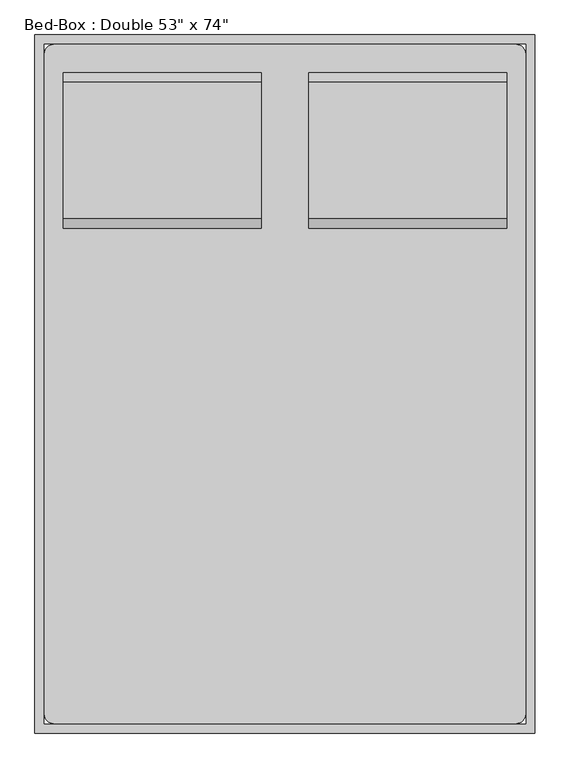
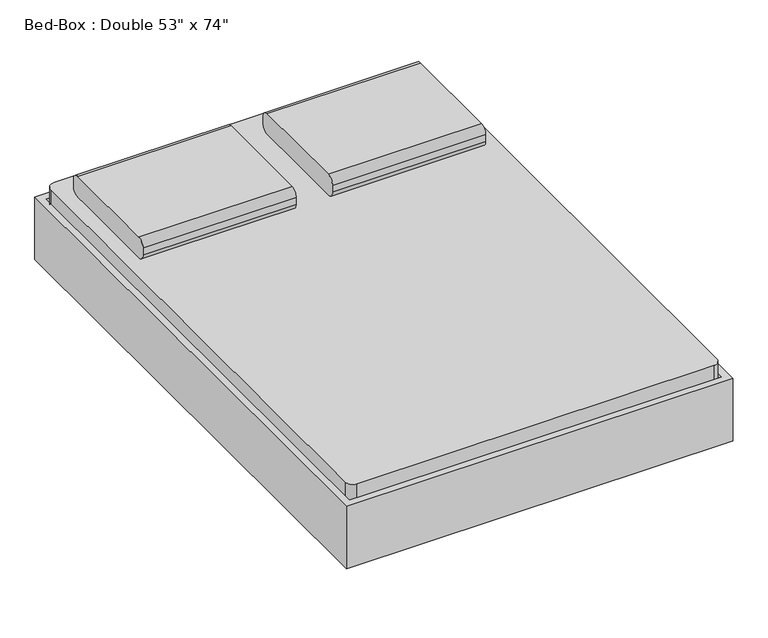
"""IFC4 building model written with IfcOpenShell, lengths in millimetres: furniture geometry."""

from ifc_helpers import new_model, si_unit, point, frame, frame_2d, origin, place, context, project, spatial, polyline, circle_curve, trimmed, segment, composite_curve, outline, extrude, source, transform, mapped, element, save
from ifc_brep_helpers import plane_surface, cylinder_surface, revolved_surface, advanced_brep


def furniture_c8abb964(model_context):
    return source(origin(), model_context, "Body", "SolidModel", [
        extrude(outline(composite_curve([segment(polyline([(578.3704918, 406.4), (210.0704918, 406.4)]), True, "CONTINUOUS"), segment(trimmed(circle_curve(frame_2d((210.0704918, 431.8)), 25.4), [point((210.0704918, 406.4))], [point((184.6704918, 431.8))], False, "CARTESIAN"), True, "CONTINUOUS"), segment(polyline([(184.6704918, 431.8), (184.6704918, 457.2)]), True, "CONTINUOUS"), segment(trimmed(circle_curve(frame_2d((210.0704918, 457.2)), 25.4), [point((184.6704918, 457.2))], [point((210.0704918, 482.6))], False, "CARTESIAN"), True, "CONTINUOUS"), segment(polyline([(210.0704918, 482.6), (578.3704918, 482.6)]), True, "CONTINUOUS"), segment(trimmed(circle_curve(frame_2d((578.3704918, 457.2)), 25.4), [point((578.3704918, 482.6))], [point((603.7704918, 457.2))], False, "CARTESIAN"), True, "CONTINUOUS"), segment(polyline([(603.7704918, 457.2), (603.7704918, 431.8)]), True, "CONTINUOUS"), segment(trimmed(circle_curve(frame_2d((578.3704918, 431.8)), 25.4), [point((603.7704918, 431.8))], [point((578.3704918, 406.4))], False, "CARTESIAN"), True, "CONTINUOUS")], self_intersect=False)), frame((402.652459, 0.0, 0.0), z_axis=(1.0, 0.0, 0.0), x_axis=(0.0, 1.0, 0.0)), (0.0, 0.0, 1.0), 533.4),
        extrude(outline(composite_curve([segment(polyline([(578.3704918, 406.4), (210.0704918, 406.4)]), True, "CONTINUOUS"), segment(trimmed(circle_curve(frame_2d((210.0704918, 431.8)), 25.4), [point((210.0704918, 406.4))], [point((184.6704918, 431.8))], False, "CARTESIAN"), True, "CONTINUOUS"), segment(polyline([(184.6704918, 431.8), (184.6704918, 457.2)]), True, "CONTINUOUS"), segment(trimmed(circle_curve(frame_2d((210.0704918, 457.2)), 25.4), [point((184.6704918, 457.2))], [point((210.0704918, 482.6))], False, "CARTESIAN"), True, "CONTINUOUS"), segment(polyline([(210.0704918, 482.6), (578.3704918, 482.6)]), True, "CONTINUOUS"), segment(trimmed(circle_curve(frame_2d((578.3704918, 457.2)), 25.4), [point((578.3704918, 482.6))], [point((603.7704918, 457.2))], False, "CARTESIAN"), True, "CONTINUOUS"), segment(polyline([(603.7704918, 457.2), (603.7704918, 431.8)]), True, "CONTINUOUS"), segment(trimmed(circle_curve(frame_2d((578.3704918, 431.8)), 25.4), [point((603.7704918, 431.8))], [point((578.3704918, 406.4))], False, "CARTESIAN"), True, "CONTINUOUS")], self_intersect=False)), frame((-257.747541, 0.0, 0.0), z_axis=(1.0, 0.0, 0.0), x_axis=(0.0, 1.0, 0.0)), (0.0, 0.0, 1.0), 533.4),
        advanced_brep(
        [(-308.2231784, 451.3704918, 177.8), (-308.2231784, 375.1704918, 177.8), (-308.2231784, 375.1704918, 196.85), (-308.2231784, 451.3704918, 196.85), (-257.4231784, 451.3704918, 177.8), (-257.4231784, 375.1704918, 177.8), (-245.2869899, 375.1704918, 196.85), (-245.2869899, 451.3704918, 196.85), (-181.3523099, 451.3704918, 14.6654962), (-181.3523099, 375.1704918, 14.6654962), (-164.0871466, 375.1704918, 22.716374), (-164.0871466, 451.3704918, 22.716374), (-158.3320921, 375.1704918, 0.0), (-158.3320921, 451.3704918, 0.0), (-158.3320921, 375.1704918, 19.05), (-158.3320921, 451.3704918, 19.05), (-79.7195862, 451.3704918, 0.0), (-79.7195862, 375.1704918, 0.0), (-79.7195862, 375.1704918, 19.05), (-79.7195862, 451.3704918, 19.05), (-67.0195862, 375.1704918, 3.4029547), (-67.0195862, 451.3704918, 3.4029547), (-76.5445862, 375.1704918, 19.9007387), (-76.5445862, 451.3704918, 19.9007387), (-6.922541, 451.3704918, 38.1), (-6.922541, 375.1704918, 38.1), (-12.0269731, 375.1704918, 57.15), (-12.0269731, 451.3704918, 57.15), (685.5518216, 451.3704918, 38.1), (685.5518216, 375.1704918, 38.1), (690.6562537, 375.1704918, 57.15), (690.6562537, 451.3704918, 57.15), (745.6488669, 451.3704918, 3.4029547), (745.6488669, 375.1704918, 3.4029547), (755.1738669, 375.1704918, 19.9007387), (755.1738669, 451.3704918, 19.9007387), (758.3488669, 375.1704918, 0.0), (758.3488669, 451.3704918, 0.0), (758.3488669, 375.1704918, 19.05), (758.3488669, 451.3704918, 19.05), (836.9613728, 451.3704918, 0.0), (836.9613728, 375.1704918, 0.0), (836.9613728, 375.1704918, 19.05), (836.9613728, 451.3704918, 19.05), (859.9815906, 375.1704918, 14.6654962), (859.9815906, 451.3704918, 14.6654962), (842.7164272, 375.1704918, 22.716374), (842.7164272, 451.3704918, 22.716374), (936.052459, 451.3704918, 177.8), (936.052459, 375.1704918, 177.8), (923.9162705, 375.1704918, 196.85), (923.9162705, 451.3704918, 196.85), (986.852459, 451.3704918, 177.8), (986.852459, 451.3704918, 196.85), (986.852459, 375.1704918, 196.85), (986.852459, 375.1704918, 177.8)],
        [
            (0, 1),
            (1, 2),
            (2, 3),
            (3, 0),
            (0, 4),
            (4, 5),
            (5, 1),
            (5, 6),
            (6, 2),
            (6, 7),
            (7, 3),
            (7, 4),
            (4, 8),
            (8, 9),
            (9, 5),
            (9, 10),
            (10, 6),
            (10, 11),
            (11, 7),
            (11, 8),
            (12, 9, circle_curve(frame((-158.3320921, 375.1704918, 25.4), z_axis=(0.0, 1.0, 0.0), x_axis=(-0.9063077870366486, 0.0, -0.42261826174070233)), 25.4)),
            (8, 13, circle_curve(frame((-158.3320921, 451.3704918, 25.4), z_axis=(0.0, -1.0, 0.0), x_axis=(-0.9063077870366486, 0.0, -0.42261826174070233)), 25.4)),
            (13, 12),
            (14, 10, circle_curve(frame((-158.3320921, 375.1704918, 25.4), z_axis=(0.0, 1.0, 0.0), x_axis=(-0.9063077870366486, 0.0, -0.42261826174070233)), 6.35)),
            (12, 14),
            (15, 11, circle_curve(frame((-158.3320921, 451.3704918, 25.4), z_axis=(0.0, 1.0, 0.0), x_axis=(-0.9063077870366486, 0.0, -0.42261826174070233)), 6.35)),
            (14, 15),
            (15, 13),
            (13, 16),
            (16, 17),
            (17, 12),
            (17, 18),
            (18, 14),
            (18, 19),
            (19, 15),
            (19, 16),
            (20, 17, circle_curve(frame((-79.7195862, 375.1704918, 25.4), z_axis=(0.0, 1.0, 0.0), x_axis=(0.0, 0.0, -1.0)), 25.4)),
            (16, 21, circle_curve(frame((-79.7195862, 451.3704918, 25.4), z_axis=(0.0, -1.0, 0.0), x_axis=(0.0, 0.0, -1.0)), 25.4)),
            (21, 20),
            (22, 18, circle_curve(frame((-79.7195862, 375.1704918, 25.4), z_axis=(0.0, 1.0, 0.0), x_axis=(0.0, 0.0, -1.0)), 6.35)),
            (20, 22),
            (23, 19, circle_curve(frame((-79.7195862, 451.3704918, 25.4), z_axis=(0.0, 1.0, 0.0), x_axis=(0.0, 0.0, -1.0)), 6.35)),
            (22, 23),
            (23, 21),
            (21, 24),
            (24, 25),
            (25, 20),
            (25, 26),
            (26, 22),
            (26, 27),
            (27, 23),
            (27, 24),
            (24, 28),
            (28, 29),
            (29, 25),
            (29, 30),
            (30, 26),
            (30, 31),
            (31, 27),
            (31, 28),
            (28, 32),
            (32, 33),
            (33, 29),
            (33, 34),
            (34, 30),
            (34, 35),
            (35, 31),
            (35, 32),
            (36, 33, circle_curve(frame((758.3488669, 375.1704918, 25.4), z_axis=(0.0, 1.0, 0.0), x_axis=(-0.5000000000000463, 0.0, -0.8660254037844118)), 25.4)),
            (32, 37, circle_curve(frame((758.3488669, 451.3704918, 25.4), z_axis=(0.0, -1.0, 0.0), x_axis=(-0.5000000000000463, 0.0, -0.8660254037844118)), 25.4)),
            (37, 36),
            (38, 34, circle_curve(frame((758.3488669, 375.1704918, 25.4), z_axis=(0.0, 1.0, 0.0), x_axis=(-0.5000000000000463, 0.0, -0.8660254037844118)), 6.35)),
            (36, 38),
            (39, 35, circle_curve(frame((758.3488669, 451.3704918, 25.4), z_axis=(0.0, 1.0, 0.0), x_axis=(-0.5000000000000463, 0.0, -0.8660254037844118)), 6.35)),
            (38, 39),
            (39, 37),
            (37, 40),
            (40, 41),
            (41, 36),
            (41, 42),
            (42, 38),
            (42, 43),
            (43, 39),
            (43, 40),
            (44, 41, circle_curve(frame((836.9613728, 375.1704918, 25.4), z_axis=(0.0, 1.0, 0.0), x_axis=(0.0, 0.0, -1.0)), 25.4)),
            (40, 45, circle_curve(frame((836.9613728, 451.3704918, 25.4), z_axis=(0.0, -1.0, 0.0), x_axis=(0.0, 0.0, -1.0)), 25.4)),
            (45, 44),
            (46, 42, circle_curve(frame((836.9613728, 375.1704918, 25.4), z_axis=(0.0, 1.0, 0.0), x_axis=(0.0, 0.0, -1.0)), 6.35)),
            (44, 46),
            (47, 43, circle_curve(frame((836.9613728, 451.3704918, 25.4), z_axis=(0.0, 1.0, 0.0), x_axis=(0.0, 0.0, -1.0)), 6.35)),
            (46, 47),
            (47, 45),
            (45, 48),
            (48, 49),
            (49, 44),
            (49, 50),
            (50, 46),
            (50, 51),
            (51, 47),
            (51, 48),
            (52, 53),
            (53, 54),
            (54, 55),
            (55, 52),
            (48, 52),
            (55, 49),
            (54, 50),
            (53, 51),
        ],
        [
            plane_surface(frame((-308.2231784, 705.3704918, -152.9490627), z_axis=(-1.0, 0.0, 0.0), x_axis=(0.0, 1.0, 0.0))),
            plane_surface(frame((-308.2231784, 451.3704918, 177.8), z_axis=(0.0, 0.0, -1.0), x_axis=(1.0, 0.0, 0.0))),
            plane_surface(frame((-308.2231784, 375.1704918, 177.8), z_axis=(0.0, -1.0, 0.0), x_axis=(1.0, 0.0, 0.0))),
            plane_surface(frame((-308.2231784, 375.1704918, 196.85), z_axis=(0.0, 0.0, 1.0), x_axis=(1.0, 0.0, 0.0))),
            plane_surface(frame((-308.2231784, 451.3704918, 196.85), z_axis=(0.0, 1.0, 0.0), x_axis=(1.0, 0.0, 0.0))),
            plane_surface(frame((-257.4231784, 451.3704918, 177.8), z_axis=(-0.9063077870366488, 0.0, -0.42261826174070194), x_axis=(0.42261826174070194, 0.0, -0.9063077870366488))),
            plane_surface(frame((-257.4231784, 375.1704918, 177.8), z_axis=(0.0, -1.0, 0.0), x_axis=(0.42261826174070194, 0.0, -0.9063077870366488))),
            plane_surface(frame((-245.2869899, 375.1704918, 196.85), z_axis=(0.9063077870366487, 0.0, 0.4226182617407021), x_axis=(0.4226182617407021, 0.0, -0.9063077870366487))),
            plane_surface(frame((-245.2869899, 451.3704918, 196.85), z_axis=(0.0, 1.0, 0.0), x_axis=(0.4226182617407021, 0.0, -0.9063077870366487))),
            cylinder_surface(frame((-158.3320921, 705.3704918, 25.4), z_axis=(0.0, -1.0, 0.0), x_axis=(-0.9063077870366486, 0.0, -0.42261826174070233)), 25.4),
            plane_surface(frame((-158.3320921, 375.1704918, 25.4), z_axis=(0.0, -1.0, 0.0), x_axis=(-0.9063077870366486, 0.0, -0.42261826174070233))),
            revolved_surface(polyline([(-164.08714654768272, 375.1704918, 22.71637403794654), (-164.08714654768272, 451.3704918, 22.71637403794654)]), (-158.3320921, 705.3704918, 25.4), (0.0, -1.0, 0.0)),
            plane_surface(frame((-158.3320921, 451.3704918, 25.4), z_axis=(0.0, 1.0, 0.0), x_axis=(-0.9063077870366486, 0.0, -0.42261826174070233))),
            plane_surface(frame((-158.3320921, 451.3704918, 0.0), z_axis=(0.0, 0.0, -1.0), x_axis=(1.0, 0.0, 0.0))),
            plane_surface(frame((-158.3320921, 375.1704918, 0.0), z_axis=(0.0, -1.0, 0.0), x_axis=(1.0, 0.0, 0.0))),
            plane_surface(frame((-158.3320921, 375.1704918, 19.05), z_axis=(0.0, 0.0, 1.0), x_axis=(1.0, 0.0, 0.0))),
            plane_surface(frame((-158.3320921, 451.3704918, 19.05), z_axis=(0.0, 1.0, 0.0), x_axis=(1.0, 0.0, 0.0))),
            cylinder_surface(frame((-79.7195862, 705.3704918, 25.4), z_axis=(0.0, -1.0, 0.0), x_axis=(0.0, 0.0, -1.0)), 25.4),
            plane_surface(frame((-79.7195862, 375.1704918, 25.4), z_axis=(0.0, -1.0, 0.0), x_axis=(0.0, 0.0, -1.0))),
            revolved_surface(polyline([(-79.7195862, 375.1704918, 19.049999999999997), (-79.7195862, 451.3704918, 19.049999999999997)]), (-79.7195862, 705.3704918, 25.4), (0.0, -1.0, 0.0)),
            plane_surface(frame((-79.7195862, 451.3704918, 25.4), z_axis=(0.0, 1.0, 0.0), x_axis=(0.0, 0.0, -1.0))),
            plane_surface(frame((-67.0195862, 451.3704918, 3.4029547), z_axis=(0.4999999999998775, 0.0, -0.8660254037845094), x_axis=(0.8660254037845094, 0.0, 0.4999999999998775))),
            plane_surface(frame((-67.0195862, 375.1704918, 3.4029547), z_axis=(0.0, -1.0, 0.0), x_axis=(0.866025403784509, 0.0, 0.49999999999987826))),
            plane_surface(frame((-76.5445862, 375.1704918, 19.9007387), z_axis=(-0.49999999999987754, 0.0, 0.8660254037845093), x_axis=(0.8660254037845093, 0.0, 0.49999999999987754))),
            plane_surface(frame((-76.5445862, 451.3704918, 19.9007387), z_axis=(0.0, 1.0000000000000002, 0.0), x_axis=(0.8660254037845091, 0.0, 0.49999999999987815))),
            plane_surface(frame((-6.922541, 451.3704918, 38.1), z_axis=(0.0, 0.0, -1.0), x_axis=(1.0, 0.0, 0.0))),
            plane_surface(frame((-6.922541, 375.1704918, 38.1), z_axis=(0.0, -1.0, 0.0), x_axis=(1.0, 0.0, 0.0))),
            plane_surface(frame((-12.0269731, 375.1704918, 57.15), z_axis=(0.0, 0.0, 1.0), x_axis=(1.0, 0.0, 0.0))),
            plane_surface(frame((-12.0269731, 451.3704918, 57.15), z_axis=(0.0, 1.0, 0.0), x_axis=(1.0, 0.0, 0.0))),
            plane_surface(frame((685.5518216, 451.3704918, 38.1), z_axis=(-0.500000000000047, 0.0, -0.8660254037844116), x_axis=(0.8660254037844116, 0.0, -0.500000000000047))),
            plane_surface(frame((685.5518216, 375.1704918, 38.1), z_axis=(0.0, -1.0, 0.0), x_axis=(0.8660254037844122, 0.0, -0.5000000000000459))),
            plane_surface(frame((690.6562537, 375.1704918, 57.15), z_axis=(0.5000000000000461, 0.0, 0.8660254037844121), x_axis=(0.8660254037844121, 0.0, -0.5000000000000461))),
            plane_surface(frame((690.6562537, 451.3704918, 57.15), z_axis=(0.0, 1.0, 0.0), x_axis=(0.8660254037844127, 0.0, -0.500000000000045))),
            cylinder_surface(frame((758.3488669, 705.3704918, 25.4), z_axis=(0.0, -1.0, 0.0), x_axis=(-0.5000000000000463, 0.0, -0.8660254037844118)), 25.4),
            plane_surface(frame((758.3488669, 375.1704918, 25.4), z_axis=(0.0, -1.0000000000000002, 0.0), x_axis=(-0.5000000000000464, 0.0, -0.866025403784412))),
            revolved_surface(polyline([(755.1738668999997, 375.1704918, 19.90073868596898), (755.1738668999997, 451.3704918, 19.90073868596898)]), (758.3488669, 705.3704918, 25.4), (0.0, -1.0, 0.0)),
            plane_surface(frame((758.3488669, 451.3704918, 25.4), z_axis=(0.0, 1.0000000000000002, 0.0), x_axis=(-0.5000000000000464, 0.0, -0.866025403784412))),
            plane_surface(frame((758.3488669, 451.3704918, 0.0), z_axis=(0.0, 0.0, -1.0), x_axis=(1.0, 0.0, 0.0))),
            plane_surface(frame((758.3488669, 375.1704918, 0.0), z_axis=(0.0, -1.0, 0.0), x_axis=(1.0, 0.0, 0.0))),
            plane_surface(frame((758.3488669, 375.1704918, 19.05), z_axis=(0.0, 0.0, 1.0), x_axis=(1.0, 0.0, 0.0))),
            plane_surface(frame((758.3488669, 451.3704918, 19.05), z_axis=(0.0, 1.0, 0.0), x_axis=(1.0, 0.0, 0.0))),
            cylinder_surface(frame((836.9613728, 705.3704918, 25.4), z_axis=(0.0, -1.0, 0.0), x_axis=(0.0, 0.0, -1.0)), 25.4),
            plane_surface(frame((836.9613728, 375.1704918, 25.4), z_axis=(0.0, -1.0, 0.0), x_axis=(0.0, 0.0, -1.0))),
            revolved_surface(polyline([(836.9613728, 375.1704918, 19.049999999999997), (836.9613728, 451.3704918, 19.049999999999997)]), (836.9613728, 705.3704918, 25.4), (0.0, -1.0, 0.0)),
            plane_surface(frame((836.9613728, 451.3704918, 25.4), z_axis=(0.0, 1.0, 0.0), x_axis=(0.0, 0.0, -1.0))),
            plane_surface(frame((859.9815906, 451.3704918, 14.6654962), z_axis=(0.9063077870366797, 0.0, -0.42261826174063566), x_axis=(0.42261826174063566, 0.0, 0.9063077870366797))),
            plane_surface(frame((859.9815906, 375.1704918, 14.6654962), z_axis=(0.0, -1.0000000000000002, 0.0), x_axis=(0.4226182617406349, 0.0, 0.9063077870366801))),
            plane_surface(frame((842.7164272, 375.1704918, 22.716374), z_axis=(-0.9063077870366799, 0.0, 0.4226182617406354), x_axis=(0.4226182617406354, 0.0, 0.9063077870366799))),
            plane_surface(frame((842.7164272, 451.3704918, 22.716374), z_axis=(0.0, 1.0, 0.0), x_axis=(0.42261826174063555, 0.0, 0.9063077870366798))),
            plane_surface(frame((986.852459, 705.3704918, -152.9490627), z_axis=(1.0, 0.0, 0.0), x_axis=(0.0, 1.0, 0.0))),
            plane_surface(frame((936.052459, 451.3704918, 177.8), z_axis=(0.0, 0.0, -1.0), x_axis=(1.0, 0.0, 0.0))),
            plane_surface(frame((936.052459, 375.1704918, 177.8), z_axis=(0.0, -1.0, 0.0), x_axis=(1.0, 0.0, 0.0))),
            plane_surface(frame((923.9162705, 375.1704918, 196.85), z_axis=(0.0, 0.0, 1.0), x_axis=(1.0, 0.0, 0.0))),
            plane_surface(frame((923.9162705, 451.3704918, 196.85), z_axis=(0.0, 1.0, 0.0), x_axis=(1.0, 0.0, 0.0))),
        ],
        [
            (0, [[1, 2, 3, 4]]),
            (1, [[-1, 5, 6, 7]]),
            (2, [[-2, -7, 8, 9]]),
            (3, [[-3, -9, 10, 11]]),
            (4, [[-4, -11, 12, -5]]),
            (5, [[-6, 13, 14, 15]]),
            (6, [[-8, -15, 16, 17]]),
            (7, [[-10, -17, 18, 19]]),
            (8, [[-12, -19, 20, -13]]),
            (9, [[21, -14, 22, 23]]),
            (10, [[24, -16, -21, 25]]),
            (11, [[26, -18, -24, 27]]),
            (12, [[-22, -20, -26, 28]]),
            (13, [[-23, 29, 30, 31]]),
            (14, [[-25, -31, 32, 33]]),
            (15, [[-27, -33, 34, 35]]),
            (16, [[-28, -35, 36, -29]]),
            (17, [[37, -30, 38, 39]]),
            (18, [[40, -32, -37, 41]]),
            (19, [[42, -34, -40, 43]]),
            (20, [[-38, -36, -42, 44]]),
            (21, [[-39, 45, 46, 47]]),
            (22, [[-41, -47, 48, 49]]),
            (23, [[-43, -49, 50, 51]]),
            (24, [[-44, -51, 52, -45]]),
            (25, [[-46, 53, 54, 55]]),
            (26, [[-48, -55, 56, 57]]),
            (27, [[-50, -57, 58, 59]]),
            (28, [[-52, -59, 60, -53]]),
            (29, [[-54, 61, 62, 63]]),
            (30, [[-56, -63, 64, 65]]),
            (31, [[-58, -65, 66, 67]]),
            (32, [[-60, -67, 68, -61]]),
            (33, [[69, -62, 70, 71]]),
            (34, [[72, -64, -69, 73]]),
            (35, [[74, -66, -72, 75]]),
            (36, [[-70, -68, -74, 76]]),
            (37, [[-71, 77, 78, 79]]),
            (38, [[-73, -79, 80, 81]]),
            (39, [[-75, -81, 82, 83]]),
            (40, [[-76, -83, 84, -77]]),
            (41, [[85, -78, 86, 87]]),
            (42, [[88, -80, -85, 89]]),
            (43, [[90, -82, -88, 91]]),
            (44, [[-86, -84, -90, 92]]),
            (45, [[-87, 93, 94, 95]]),
            (46, [[-89, -95, 96, 97]]),
            (47, [[-91, -97, 98, 99]]),
            (48, [[-92, -99, 100, -93]]),
            (49, [[101, 102, 103, 104]]),
            (50, [[-94, 105, -104, 106]]),
            (51, [[-96, -106, -103, 107]]),
            (52, [[-98, -107, -102, 108]]),
            (53, [[-100, -108, -101, -105]]),
        ],
    ),
        extrude(outline(composite_curve([segment(polyline([(-283.147541, 679.9704918), (961.452459, 679.9704918)]), True, "CONTINUOUS"), segment(trimmed(circle_curve(frame_2d((961.452459, 654.5704918)), 25.4), [point((961.452459, 679.9704918))], [point((986.852459, 654.5704918))], False, "CARTESIAN"), True, "CONTINUOUS"), segment(polyline([(986.852459, 654.5704918), (986.852459, -1123.4295082)]), True, "CONTINUOUS"), segment(trimmed(circle_curve(frame_2d((961.452459, -1123.4295082)), 25.4), [point((986.852459, -1123.4295082))], [point((961.452459, -1148.8295082))], False, "CARTESIAN"), True, "CONTINUOUS"), segment(polyline([(961.452459, -1148.8295082), (-283.147541, -1148.8295082)]), True, "CONTINUOUS"), segment(trimmed(circle_curve(frame_2d((-283.147541, -1123.4295082)), 25.4), [point((-283.147541, -1148.8295082))], [point((-308.547541, -1123.4295082))], False, "CARTESIAN"), True, "CONTINUOUS"), segment(polyline([(-308.547541, -1123.4295082), (-308.547541, 654.5704918)]), True, "CONTINUOUS"), segment(trimmed(circle_curve(frame_2d((-283.147541, 654.5704918)), 25.4), [point((-308.547541, 654.5704918))], [point((-283.147541, 679.9704918))], False, "CARTESIAN"), True, "CONTINUOUS")], self_intersect=False)), frame((0.0, 0.0, 203.2), z_axis=(0.0, 0.0, 1.0), x_axis=(1.0, 0.0, 0.0)), (0.0, 0.0, 1.0), 203.2),
        advanced_brep(
        [(-308.547541, -869.4295082, 196.85), (-308.547541, -869.4295082, 177.8), (-308.547541, -945.6295082, 177.8), (-308.547541, -945.6295082, 196.85), (-245.6113525, -869.4295082, 196.85), (-257.747541, -869.4295082, 177.8), (-257.747541, -945.6295082, 177.8), (-245.6113525, -945.6295082, 196.85), (-164.4115092, -869.4295082, 22.716374), (-181.6766725, -869.4295082, 14.6654962), (-181.6766725, -945.6295082, 14.6654962), (-164.4115092, -945.6295082, 22.716374), (-158.6564547, -869.4295082, 0.0), (-158.6564547, -869.4295082, 19.05), (-158.6564547, -945.6295082, 0.0), (-158.6564547, -945.6295082, 19.05), (-80.0439489, -869.4295082, 19.05), (-80.0439489, -869.4295082, 0.0), (-80.0439489, -945.6295082, 0.0), (-80.0439489, -945.6295082, 19.05), (-67.3439489, -869.4295082, 3.4029547), (-76.8689489, -869.4295082, 19.9007387), (-67.3439489, -945.6295082, 3.4029547), (-76.8689489, -945.6295082, 19.9007387), (-12.3513357, -869.4295082, 57.15), (-7.2469036, -869.4295082, 38.1), (-7.2469036, -945.6295082, 38.1), (-12.3513357, -945.6295082, 57.15), (690.6562537, -869.4295082, 57.15), (685.5518216, -869.4295082, 38.1), (685.5518216, -945.6295082, 38.1), (690.6562537, -945.6295082, 57.15), (755.1738669, -869.4295082, 19.9007387), (745.6488669, -869.4295082, 3.4029547), (745.6488669, -945.6295082, 3.4029547), (755.1738669, -945.6295082, 19.9007387), (758.3488669, -869.4295082, 0.0), (758.3488669, -869.4295082, 19.05), (758.3488669, -945.6295082, 0.0), (758.3488669, -945.6295082, 19.05), (836.9613728, -869.4295082, 19.05), (836.9613728, -869.4295082, 0.0), (836.9613728, -945.6295082, 0.0), (836.9613728, -945.6295082, 19.05), (859.9815906, -869.4295082, 14.6654962), (842.7164272, -869.4295082, 22.716374), (859.9815906, -945.6295082, 14.6654962), (842.7164272, -945.6295082, 22.716374), (923.9162705, -869.4295082, 196.85), (936.052459, -869.4295082, 177.8), (936.052459, -945.6295082, 177.8), (923.9162705, -945.6295082, 196.85), (986.852459, -869.4295082, 196.85), (986.852459, -945.6295082, 196.85), (986.852459, -945.6295082, 177.8), (986.852459, -869.4295082, 177.8)],
        [
            (0, 1),
            (1, 2),
            (2, 3),
            (3, 0),
            (0, 4),
            (4, 5),
            (5, 1),
            (5, 6),
            (6, 2),
            (6, 7),
            (7, 3),
            (7, 4),
            (4, 8),
            (8, 9),
            (9, 5),
            (9, 10),
            (10, 6),
            (10, 11),
            (11, 7),
            (11, 8),
            (12, 9, circle_curve(frame((-158.6564547, -869.4295082, 25.4), z_axis=(0.0, 1.0, 0.0), x_axis=(-0.906307787036663, 0.0, -0.4226182617406713)), 25.4)),
            (8, 13, circle_curve(frame((-158.6564547, -869.4295082, 25.4), z_axis=(0.0, -1.0, 0.0), x_axis=(-0.906307787036663, 0.0, -0.4226182617406713)), 6.35)),
            (13, 12),
            (14, 10, circle_curve(frame((-158.6564547, -945.6295082, 25.4), z_axis=(0.0, 1.0, 0.0), x_axis=(-0.906307787036663, 0.0, -0.4226182617406713)), 25.4)),
            (12, 14),
            (15, 11, circle_curve(frame((-158.6564547, -945.6295082, 25.4), z_axis=(0.0, 1.0, 0.0), x_axis=(-0.906307787036663, 0.0, -0.4226182617406713)), 6.35)),
            (14, 15),
            (15, 13),
            (13, 16),
            (16, 17),
            (17, 12),
            (17, 18),
            (18, 14),
            (18, 19),
            (19, 15),
            (19, 16),
            (20, 17, circle_curve(frame((-80.0439489, -869.4295082, 25.4), z_axis=(0.0, 1.0, 0.0), x_axis=(0.0, 0.0, -1.0)), 25.4)),
            (16, 21, circle_curve(frame((-80.0439489, -869.4295082, 25.4), z_axis=(0.0, -1.0, 0.0), x_axis=(0.0, 0.0, -1.0)), 6.35)),
            (21, 20),
            (22, 18, circle_curve(frame((-80.0439489, -945.6295082, 25.4), z_axis=(0.0, 1.0, 0.0), x_axis=(0.0, 0.0, -1.0)), 25.4)),
            (20, 22),
            (23, 19, circle_curve(frame((-80.0439489, -945.6295082, 25.4), z_axis=(0.0, 1.0, 0.0), x_axis=(0.0, 0.0, -1.0)), 6.35)),
            (22, 23),
            (23, 21),
            (21, 24),
            (24, 25),
            (25, 20),
            (25, 26),
            (26, 22),
            (26, 27),
            (27, 23),
            (27, 24),
            (24, 28),
            (28, 29),
            (29, 25),
            (29, 30),
            (30, 26),
            (30, 31),
            (31, 27),
            (31, 28),
            (28, 32),
            (32, 33),
            (33, 29),
            (33, 34),
            (34, 30),
            (34, 35),
            (35, 31),
            (35, 32),
            (36, 33, circle_curve(frame((758.3488669, -869.4295082, 25.4), z_axis=(0.0, 1.0, 0.0), x_axis=(-0.5000000000000479, 0.0, -0.866025403784411)), 25.4)),
            (32, 37, circle_curve(frame((758.3488669, -869.4295082, 25.4), z_axis=(0.0, -1.0, 0.0), x_axis=(-0.5000000000000479, 0.0, -0.866025403784411)), 6.35)),
            (37, 36),
            (38, 34, circle_curve(frame((758.3488669, -945.6295082, 25.4), z_axis=(0.0, 1.0, 0.0), x_axis=(-0.5000000000000479, 0.0, -0.866025403784411)), 25.4)),
            (36, 38),
            (39, 35, circle_curve(frame((758.3488669, -945.6295082, 25.4), z_axis=(0.0, 1.0, 0.0), x_axis=(-0.5000000000000479, 0.0, -0.866025403784411)), 6.35)),
            (38, 39),
            (39, 37),
            (37, 40),
            (40, 41),
            (41, 36),
            (41, 42),
            (42, 38),
            (42, 43),
            (43, 39),
            (43, 40),
            (44, 41, circle_curve(frame((836.9613728, -869.4295082, 25.4), z_axis=(0.0, 1.0, 0.0), x_axis=(0.0, 0.0, -1.0)), 25.4)),
            (40, 45, circle_curve(frame((836.9613728, -869.4295082, 25.4), z_axis=(0.0, -1.0, 0.0), x_axis=(0.0, 0.0, -1.0)), 6.35)),
            (45, 44),
            (46, 42, circle_curve(frame((836.9613728, -945.6295082, 25.4), z_axis=(0.0, 1.0, 0.0), x_axis=(0.0, 0.0, -1.0)), 25.4)),
            (44, 46),
            (47, 43, circle_curve(frame((836.9613728, -945.6295082, 25.4), z_axis=(0.0, 1.0, 0.0), x_axis=(0.0, 0.0, -1.0)), 6.35)),
            (46, 47),
            (47, 45),
            (45, 48),
            (48, 49),
            (49, 44),
            (49, 50),
            (50, 46),
            (50, 51),
            (51, 47),
            (51, 48),
            (52, 53),
            (53, 54),
            (54, 55),
            (55, 52),
            (48, 52),
            (55, 49),
            (54, 50),
            (53, 51),
        ],
        [
            plane_surface(frame((-308.547541, -1174.2295082, -127.5947323), z_axis=(-1.0, 0.0, 0.0), x_axis=(0.0, 1.0, 0.0))),
            plane_surface(frame((-308.547541, -869.4295082, 196.85), z_axis=(0.0, 1.0, 0.0), x_axis=(1.0, 0.0, 0.0))),
            plane_surface(frame((-308.547541, -869.4295082, 177.8), z_axis=(0.0, 0.0, -1.0), x_axis=(1.0, 0.0, 0.0))),
            plane_surface(frame((-308.547541, -945.6295082, 177.8), z_axis=(0.0, -1.0, 0.0), x_axis=(1.0, 0.0, 0.0))),
            plane_surface(frame((-308.547541, -945.6295082, 196.85), z_axis=(0.0, 0.0, 1.0), x_axis=(1.0, 0.0, 0.0))),
            plane_surface(frame((-245.6113525, -869.4295082, 196.85), z_axis=(0.0, 1.0, 0.0), x_axis=(0.422618261740671, 0.0, -0.9063077870366633))),
            plane_surface(frame((-257.747541, -869.4295082, 177.8), z_axis=(-0.9063077870366631, 0.0, -0.42261826174067113), x_axis=(0.42261826174067113, 0.0, -0.9063077870366631))),
            plane_surface(frame((-257.747541, -945.6295082, 177.8), z_axis=(0.0, -1.0, 0.0), x_axis=(0.42261826174067135, 0.0, -0.906307787036663))),
            plane_surface(frame((-245.6113525, -945.6295082, 196.85), z_axis=(0.9063077870366631, 0.0, 0.4226182617406713), x_axis=(0.4226182617406713, 0.0, -0.9063077870366631))),
            plane_surface(frame((-158.6564547, -869.4295082, 25.4), z_axis=(0.0, 1.0, 0.0), x_axis=(-0.906307787036663, 0.0, -0.4226182617406713))),
            cylinder_surface(frame((-158.6564547, -1174.2295082, 25.4), z_axis=(0.0, -1.0, 0.0), x_axis=(-0.906307787036663, 0.0, -0.4226182617406713)), 25.4),
            plane_surface(frame((-158.6564547, -945.6295082, 25.4), z_axis=(0.0, -1.0, 0.0), x_axis=(-0.906307787036663, 0.0, -0.4226182617406713))),
            revolved_surface(polyline([(-164.41150914768284, -945.6295082, 22.716374037946736), (-164.41150914768284, -869.4295082, 22.716374037946736)]), (-158.6564547, -1174.2295082, 25.4), (0.0, -1.0, 0.0)),
            plane_surface(frame((-158.6564547, -869.4295082, 19.05), z_axis=(0.0, 1.0, 0.0), x_axis=(1.0, 0.0, 0.0))),
            plane_surface(frame((-158.6564547, -869.4295082, 0.0), z_axis=(0.0, 0.0, -1.0), x_axis=(1.0, 0.0, 0.0))),
            plane_surface(frame((-158.6564547, -945.6295082, 0.0), z_axis=(0.0, -1.0, 0.0), x_axis=(1.0, 0.0, 0.0))),
            plane_surface(frame((-158.6564547, -945.6295082, 19.05), z_axis=(0.0, 0.0, 1.0), x_axis=(1.0, 0.0, 0.0))),
            plane_surface(frame((-80.0439489, -869.4295082, 25.4), z_axis=(0.0, 1.0, 0.0), x_axis=(0.0, 0.0, -1.0))),
            cylinder_surface(frame((-80.0439489, -1174.2295082, 25.4), z_axis=(0.0, -1.0, 0.0), x_axis=(0.0, 0.0, -1.0)), 25.4),
            plane_surface(frame((-80.0439489, -945.6295082, 25.4), z_axis=(0.0, -1.0, 0.0), x_axis=(0.0, 0.0, -1.0))),
            revolved_surface(polyline([(-80.0439489, -945.6295082, 19.049999999999997), (-80.0439489, -869.4295082, 19.049999999999997)]), (-80.0439489, -1174.2295082, 25.4), (0.0, -1.0, 0.0)),
            plane_surface(frame((-76.8689489, -869.4295082, 19.9007387), z_axis=(0.0, 1.0, 0.0), x_axis=(0.8660254037844785, 0.0, 0.499999999999931))),
            plane_surface(frame((-67.3439489, -869.4295082, 3.4029547), z_axis=(0.499999999999931, 0.0, -0.8660254037844785), x_axis=(0.8660254037844785, 0.0, 0.499999999999931))),
            plane_surface(frame((-67.3439489, -945.6295082, 3.4029547), z_axis=(0.0, -1.0, 0.0), x_axis=(0.8660254037844786, 0.0, 0.49999999999993094))),
            plane_surface(frame((-76.8689489, -945.6295082, 19.9007387), z_axis=(-0.4999999999999312, 0.0, 0.8660254037844785), x_axis=(0.8660254037844785, 0.0, 0.4999999999999312))),
            plane_surface(frame((-12.3513357, -869.4295082, 57.15), z_axis=(0.0, 1.0, 0.0), x_axis=(1.0, 0.0, 0.0))),
            plane_surface(frame((-7.2469036, -869.4295082, 38.1), z_axis=(0.0, 0.0, -1.0), x_axis=(1.0, 0.0, 0.0))),
            plane_surface(frame((-7.2469036, -945.6295082, 38.1), z_axis=(0.0, -1.0, 0.0), x_axis=(1.0, 0.0, 0.0))),
            plane_surface(frame((-12.3513357, -945.6295082, 57.15), z_axis=(0.0, 0.0, 1.0), x_axis=(1.0, 0.0, 0.0))),
            plane_surface(frame((690.6562537, -869.4295082, 57.15), z_axis=(0.0, 1.0, 0.0), x_axis=(0.8660254037844091, 0.0, -0.5000000000000514))),
            plane_surface(frame((685.5518216, -869.4295082, 38.1), z_axis=(-0.5000000000000502, 0.0, -0.8660254037844097), x_axis=(0.8660254037844097, 0.0, -0.5000000000000502))),
            plane_surface(frame((685.5518216, -945.6295082, 38.1), z_axis=(0.0, -1.0, 0.0), x_axis=(0.86602540378441, 0.0, -0.5000000000000498))),
            plane_surface(frame((690.6562537, -945.6295082, 57.15), z_axis=(0.5000000000000505, 0.0, 0.8660254037844095), x_axis=(0.8660254037844095, 0.0, -0.5000000000000505))),
            plane_surface(frame((758.3488669, -869.4295082, 25.4), z_axis=(0.0, 1.0000000000000002, 0.0), x_axis=(-0.500000000000048, 0.0, -0.8660254037844111))),
            cylinder_surface(frame((758.3488669, -1174.2295082, 25.4), z_axis=(0.0, -1.0, 0.0), x_axis=(-0.5000000000000479, 0.0, -0.866025403784411)), 25.4),
            plane_surface(frame((758.3488669, -945.6295082, 25.4), z_axis=(0.0, -1.0000000000000002, 0.0), x_axis=(-0.500000000000048, 0.0, -0.8660254037844111))),
            revolved_surface(polyline([(755.1738668999997, -945.6295082, 19.90073868596899), (755.1738668999997, -869.4295082, 19.90073868596899)]), (758.3488669, -1174.2295082, 25.4), (0.0, -1.0, 0.0)),
            plane_surface(frame((758.3488669, -869.4295082, 19.05), z_axis=(0.0, 1.0, 0.0), x_axis=(1.0, 0.0, 0.0))),
            plane_surface(frame((758.3488669, -869.4295082, 0.0), z_axis=(0.0, 0.0, -1.0), x_axis=(1.0, 0.0, 0.0))),
            plane_surface(frame((758.3488669, -945.6295082, 0.0), z_axis=(0.0, -1.0, 0.0), x_axis=(1.0, 0.0, 0.0))),
            plane_surface(frame((758.3488669, -945.6295082, 19.05), z_axis=(0.0, 0.0, 1.0), x_axis=(1.0, 0.0, 0.0))),
            plane_surface(frame((836.9613728, -869.4295082, 25.4), z_axis=(0.0, 1.0, 0.0), x_axis=(0.0, 0.0, -1.0))),
            cylinder_surface(frame((836.9613728, -1174.2295082, 25.4), z_axis=(0.0, -1.0, 0.0), x_axis=(0.0, 0.0, -1.0)), 25.4),
            plane_surface(frame((836.9613728, -945.6295082, 25.4), z_axis=(0.0, -1.0, 0.0), x_axis=(0.0, 0.0, -1.0))),
            revolved_surface(polyline([(836.9613728, -945.6295082, 19.049999999999997), (836.9613728, -869.4295082, 19.049999999999997)]), (836.9613728, -1174.2295082, 25.4), (0.0, -1.0, 0.0)),
            plane_surface(frame((842.7164272, -869.4295082, 22.716374), z_axis=(0.0, 1.0, 0.0), x_axis=(0.4226182617405411, 0.0, 0.9063077870367238))),
            plane_surface(frame((859.9815906, -869.4295082, 14.6654962), z_axis=(0.9063077870367237, 0.0, -0.42261826174054157), x_axis=(0.42261826174054157, 0.0, 0.9063077870367237))),
            plane_surface(frame((859.9815906, -945.6295082, 14.6654962), z_axis=(0.0, -1.0, 0.0), x_axis=(0.4226182617405412, 0.0, 0.9063077870367238))),
            plane_surface(frame((842.7164272, -945.6295082, 22.716374), z_axis=(-0.906307787036724, 0.0, 0.422618261740541), x_axis=(0.422618261740541, 0.0, 0.906307787036724))),
            plane_surface(frame((986.852459, -1174.2295082, -127.5947323), z_axis=(1.0, 0.0, 0.0), x_axis=(0.0, 1.0, 0.0))),
            plane_surface(frame((923.9162705, -869.4295082, 196.85), z_axis=(0.0, 1.0, 0.0), x_axis=(1.0, 0.0, 0.0))),
            plane_surface(frame((936.052459, -869.4295082, 177.8), z_axis=(0.0, 0.0, -1.0), x_axis=(1.0, 0.0, 0.0))),
            plane_surface(frame((936.052459, -945.6295082, 177.8), z_axis=(0.0, -1.0, 0.0), x_axis=(1.0, 0.0, 0.0))),
            plane_surface(frame((923.9162705, -945.6295082, 196.85), z_axis=(0.0, 0.0, 1.0), x_axis=(1.0, 0.0, 0.0))),
        ],
        [
            (0, [[1, 2, 3, 4]]),
            (1, [[-1, 5, 6, 7]]),
            (2, [[-2, -7, 8, 9]]),
            (3, [[-3, -9, 10, 11]]),
            (4, [[-4, -11, 12, -5]]),
            (5, [[-6, 13, 14, 15]]),
            (6, [[-8, -15, 16, 17]]),
            (7, [[-10, -17, 18, 19]]),
            (8, [[-12, -19, 20, -13]]),
            (9, [[21, -14, 22, 23]]),
            (10, [[24, -16, -21, 25]]),
            (11, [[26, -18, -24, 27]]),
            (12, [[-22, -20, -26, 28]]),
            (13, [[-23, 29, 30, 31]]),
            (14, [[-25, -31, 32, 33]]),
            (15, [[-27, -33, 34, 35]]),
            (16, [[-28, -35, 36, -29]]),
            (17, [[37, -30, 38, 39]]),
            (18, [[40, -32, -37, 41]]),
            (19, [[42, -34, -40, 43]]),
            (20, [[-38, -36, -42, 44]]),
            (21, [[-39, 45, 46, 47]]),
            (22, [[-41, -47, 48, 49]]),
            (23, [[-43, -49, 50, 51]]),
            (24, [[-44, -51, 52, -45]]),
            (25, [[-46, 53, 54, 55]]),
            (26, [[-48, -55, 56, 57]]),
            (27, [[-50, -57, 58, 59]]),
            (28, [[-52, -59, 60, -53]]),
            (29, [[-54, 61, 62, 63]]),
            (30, [[-56, -63, 64, 65]]),
            (31, [[-58, -65, 66, 67]]),
            (32, [[-60, -67, 68, -61]]),
            (33, [[69, -62, 70, 71]]),
            (34, [[72, -64, -69, 73]]),
            (35, [[74, -66, -72, 75]]),
            (36, [[-70, -68, -74, 76]]),
            (37, [[-71, 77, 78, 79]]),
            (38, [[-73, -79, 80, 81]]),
            (39, [[-75, -81, 82, 83]]),
            (40, [[-76, -83, 84, -77]]),
            (41, [[85, -78, 86, 87]]),
            (42, [[88, -80, -85, 89]]),
            (43, [[90, -82, -88, 91]]),
            (44, [[-86, -84, -90, 92]]),
            (45, [[-87, 93, 94, 95]]),
            (46, [[-89, -95, 96, 97]]),
            (47, [[-91, -97, 98, 99]]),
            (48, [[-92, -99, 100, -93]]),
            (49, [[101, 102, 103, 104]]),
            (50, [[-94, 105, -104, 106]]),
            (51, [[-96, -106, -103, 107]]),
            (52, [[-98, -107, -102, 108]]),
            (53, [[-100, -108, -101, -105]]),
        ],
    ),
        extrude(outline(polyline([(1012.252459, 705.3704918), (1012.252459, -1174.2295082), (-333.947541, -1174.2295082), (-333.947541, 705.3704918), (1012.252459, 705.3704918)]), holes=[polyline([(986.852459, 679.9704918), (-308.547541, 679.9704918), (-308.547541, -1148.8295082), (986.852459, -1148.8295082), (986.852459, 679.9704918)])]), frame((0.0, 0.0, 127.0), z_axis=(0.0, 0.0, 1.0), x_axis=(1.0, 0.0, 0.0)), (0.0, 0.0, 1.0), 228.6),
    ])


if __name__ == "__main__":
    model = new_model("IFC4")
    model_context = context("Model", 3, world=origin())
    ifc_project = project(units=[si_unit("LENGTHUNIT", "METRE", prefix="MILLI")], contexts=[model_context])
    site = spatial("IfcSite", under=ifc_project)
    building = spatial("IfcBuilding", under=site)
    placement = place(None, origin())
    furniture_shape = furniture_c8abb964(model_context)
    element("IfcFurniture", 1, ObjectType="Bed-Box : Double 53\" x 74\"", at=placement, inside=building, context=model_context, shape_type="MappedRepresentation", body=[
        mapped(furniture_shape, transform((0.0, 0.0, 0.0), x_axis=(1.0, 0.0, 0.0), y_axis=(0.0, 1.0, 0.0), z_axis=(0.0, 0.0, 1.0))),
    ])
    save(model, "model.ifc")

# Revit data of these elements
# Type "Bed-Box : Double 53\" x 74\""
#   Assembly Code = "E2020200"
#   Length = 6' - 2"
#   Width = 4' - 5"
#   Frame Material = Sash
#   Mattress Material = Sash
#   Default Elevation = 0
# Element 1 (IfcFurniture, "Bed-Box : Double 53\" x 74\"")
#   Materials on its faces: "Sash"
# Materials
#   "Sash": class "Wood", colour RGB 224 178 126, transparency 0
